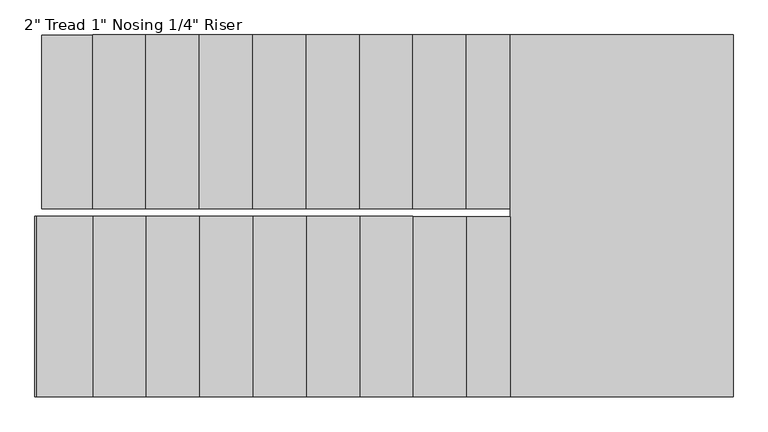
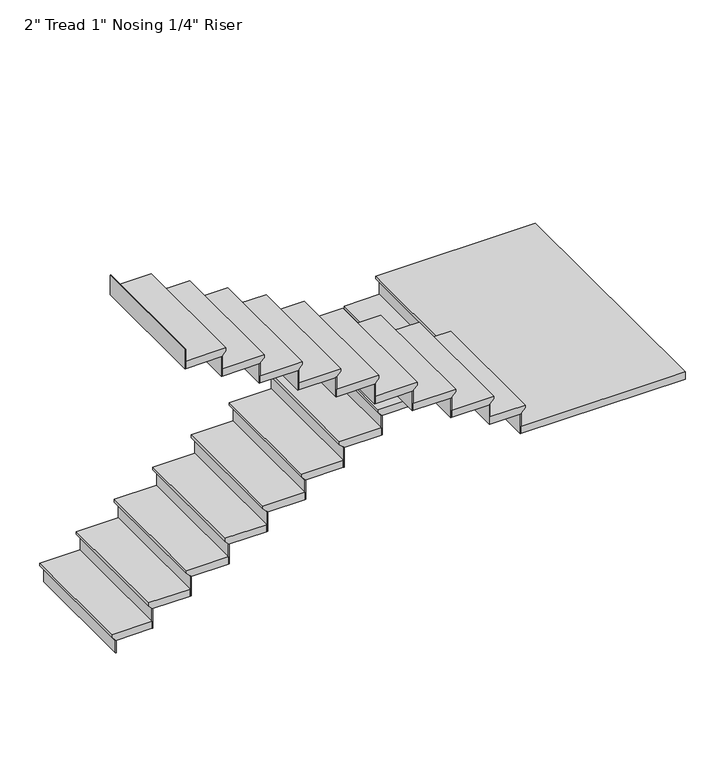
"""IFC4 building model written with IfcOpenShell, lengths in millimetres: stair flight geometry."""

from ifc_helpers import new_model, si_unit, origin, place, context, project, spatial, faceted_brep, source, transform, mapped, element, save


def stair_flight_b1286695(model_context):
    return source(origin(), model_context, "Body", "Brep", [
        faceted_brep([(1537.1941283, 180.9547293, 9262.11), (1537.1941283, 180.9547293, 9281.16), (1537.1941283, 1006.4547293, 9281.16), (1537.1941283, 1006.4547293, 9262.11), (1562.5941283, 180.9547293, 9236.71), (1562.5941283, 1006.4547293, 9236.71), (1804.8381368, 180.9547293, 9281.16), (1804.8381368, 1006.4547293, 9281.16), (1562.5941283, 1006.4547293, 9230.36), (1804.8381368, 1006.4547293, 9230.36), (1804.8381368, 180.9547293, 9230.36), (1562.5941283, 180.9547293, 9230.36)], [[[0, 1, 2, 3]], [[4, 0, 3, 5]], [[2, 1, 6, 7]], [[8, 9, 10, 11]], [[2, 7, 9, 8, 5, 3]], [[8, 11, 4, 5]], [[6, 1, 0, 4, 11, 10]], [[7, 6, 10, 9]]]),
        faceted_brep([(1562.5941283, 180.9547293, 9230.36), (1562.5941283, 180.9547293, 9144.0), (1568.9441283, 180.9547293, 9144.0), (1568.9441283, 180.9547293, 9230.36), (1562.5941283, 1006.4547293, 9230.36), (1568.9441283, 1006.4547293, 9230.36), (1568.9441283, 1006.4547293, 9144.0), (1562.5941283, 1006.4547293, 9144.0)], [[[0, 1, 2, 3]], [[4, 5, 6, 7]], [[1, 0, 4, 7]], [[2, 1, 7, 6]], [[3, 2, 6, 5]], [[0, 3, 5, 4]]]),
        faceted_brep([(1804.8381368, 180.9547293, 9367.52), (1804.8381368, 180.9547293, 9230.36), (1811.1881368, 180.9547293, 9230.36), (1811.1881368, 180.9547293, 9367.52), (1804.8381368, 1006.4547293, 9367.52), (1811.1881368, 1006.4547293, 9367.52), (1811.1881368, 1006.4547293, 9230.36), (1804.8381368, 1006.4547293, 9230.36)], [[[0, 1, 2, 3]], [[4, 5, 6, 7]], [[1, 0, 4, 7]], [[2, 1, 7, 6]], [[3, 2, 6, 5]], [[0, 3, 5, 4]]]),
        faceted_brep([(1779.4381368, 1006.4547293, 9418.32), (1779.4381368, 180.9547293, 9418.32), (2058.8381368, 180.9547293, 9418.32), (2058.8381368, 1006.4547293, 9418.32), (1804.8381368, 1006.4547293, 9367.52), (2058.8381368, 1006.4547293, 9367.52), (2058.8381368, 180.9547293, 9367.52), (1804.8381368, 180.9547293, 9367.52), (1804.8381368, 1006.4547293, 9373.87), (1779.4381368, 1006.4547293, 9399.27), (1804.8381368, 180.9547293, 9373.87), (1779.4381368, 180.9547293, 9399.27)], [[[0, 1, 2, 3]], [[4, 5, 6, 7]], [[0, 3, 5, 4, 8, 9]], [[4, 7, 10, 8]], [[2, 1, 11, 10, 7, 6]], [[3, 2, 6, 5]], [[11, 1, 0, 9]], [[10, 11, 9, 8]]]),
        faceted_brep([(2058.8381368, 180.9547293, 9504.68), (2058.8381368, 180.9547293, 9367.52), (2065.1881368, 180.9547293, 9367.52), (2065.1881368, 180.9547293, 9504.68), (2058.8381368, 1006.4547293, 9504.68), (2065.1881368, 1006.4547293, 9504.68), (2065.1881368, 1006.4547293, 9367.52), (2058.8381368, 1006.4547293, 9367.52)], [[[0, 1, 2, 3]], [[4, 5, 6, 7]], [[1, 0, 4, 7]], [[2, 1, 7, 6]], [[3, 2, 6, 5]], [[0, 3, 5, 4]]]),
        faceted_brep([(2033.4381368, 1006.4547293, 9555.48), (2033.4381368, 180.9547293, 9555.48), (2312.8381368, 180.9547293, 9555.48), (2312.8381368, 1006.4547293, 9555.48), (2058.8381368, 1006.4547293, 9504.68), (2312.8381368, 1006.4547293, 9504.68), (2312.8381368, 180.9547293, 9504.68), (2058.8381368, 180.9547293, 9504.68), (2058.8381368, 1006.4547293, 9511.03), (2033.4381368, 1006.4547293, 9536.43), (2058.8381368, 180.9547293, 9511.03), (2033.4381368, 180.9547293, 9536.43)], [[[0, 1, 2, 3]], [[4, 5, 6, 7]], [[0, 3, 5, 4, 8, 9]], [[4, 7, 10, 8]], [[2, 1, 11, 10, 7, 6]], [[3, 2, 6, 5]], [[11, 1, 0, 9]], [[10, 11, 9, 8]]]),
        faceted_brep([(2312.8381368, 180.9547293, 9641.84), (2312.8381368, 180.9547293, 9504.68), (2319.1881368, 180.9547293, 9504.68), (2319.1881368, 180.9547293, 9641.84), (2312.8381368, 1006.4547293, 9641.84), (2319.1881368, 1006.4547293, 9641.84), (2319.1881368, 1006.4547293, 9504.68), (2312.8381368, 1006.4547293, 9504.68)], [[[0, 1, 2, 3]], [[4, 5, 6, 7]], [[1, 0, 4, 7]], [[2, 1, 7, 6]], [[3, 2, 6, 5]], [[0, 3, 5, 4]]]),
        faceted_brep([(2287.4381368, 1006.4547293, 9692.64), (2287.4381368, 180.9547293, 9692.64), (2566.8381368, 180.9547293, 9692.64), (2566.8381368, 1006.4547293, 9692.64), (2312.8381368, 1006.4547293, 9641.84), (2566.8381368, 1006.4547293, 9641.84), (2566.8381368, 180.9547293, 9641.84), (2312.8381368, 180.9547293, 9641.84), (2312.8381368, 1006.4547293, 9648.19), (2287.4381368, 1006.4547293, 9673.59), (2312.8381368, 180.9547293, 9648.19), (2287.4381368, 180.9547293, 9673.59)], [[[0, 1, 2, 3]], [[4, 5, 6, 7]], [[0, 3, 5, 4, 8, 9]], [[4, 7, 10, 8]], [[2, 1, 11, 10, 7, 6]], [[3, 2, 6, 5]], [[11, 1, 0, 9]], [[10, 11, 9, 8]]]),
        faceted_brep([(2566.8381368, 180.9547293, 9779.0), (2566.8381368, 180.9547293, 9641.84), (2573.1881368, 180.9547293, 9641.84), (2573.1881368, 180.9547293, 9779.0), (2566.8381368, 1006.4547293, 9779.0), (2573.1881368, 1006.4547293, 9779.0), (2573.1881368, 1006.4547293, 9641.84), (2566.8381368, 1006.4547293, 9641.84)], [[[0, 1, 2, 3]], [[4, 5, 6, 7]], [[1, 0, 4, 7]], [[2, 1, 7, 6]], [[3, 2, 6, 5]], [[0, 3, 5, 4]]]),
        faceted_brep([(2541.4381368, 1006.4547293, 9829.8), (2541.4381368, 180.9547293, 9829.8), (2820.8381368, 180.9547293, 9829.8), (2820.8381368, 1006.4547293, 9829.8), (2566.8381368, 1006.4547293, 9779.0), (2820.8381368, 1006.4547293, 9779.0), (2820.8381368, 180.9547293, 9779.0), (2566.8381368, 180.9547293, 9779.0), (2566.8381368, 1006.4547293, 9785.35), (2541.4381368, 1006.4547293, 9810.75), (2566.8381368, 180.9547293, 9785.35), (2541.4381368, 180.9547293, 9810.75)], [[[0, 1, 2, 3]], [[4, 5, 6, 7]], [[0, 3, 5, 4, 8, 9]], [[4, 7, 10, 8]], [[2, 1, 11, 10, 7, 6]], [[3, 2, 6, 5]], [[11, 1, 0, 9]], [[10, 11, 9, 8]]]),
        faceted_brep([(2820.8381368, 180.9547293, 9916.16), (2820.8381368, 180.9547293, 9779.0), (2827.1881368, 180.9547293, 9779.0), (2827.1881368, 180.9547293, 9916.16), (2820.8381368, 1006.4547293, 9916.16), (2827.1881368, 1006.4547293, 9916.16), (2827.1881368, 1006.4547293, 9779.0), (2820.8381368, 1006.4547293, 9779.0)], [[[0, 1, 2, 3]], [[4, 5, 6, 7]], [[1, 0, 4, 7]], [[2, 1, 7, 6]], [[3, 2, 6, 5]], [[0, 3, 5, 4]]]),
        faceted_brep([(2795.4381368, 1006.4547293, 9966.96), (2795.4381368, 180.9547293, 9966.96), (3074.8381368, 180.9547293, 9966.96), (3074.8381368, 1006.4547293, 9966.96), (2820.8381368, 1006.4547293, 9916.16), (3074.8381368, 1006.4547293, 9916.16), (3074.8381368, 180.9547293, 9916.16), (2820.8381368, 180.9547293, 9916.16), (2820.8381368, 1006.4547293, 9922.51), (2795.4381368, 1006.4547293, 9947.91), (2820.8381368, 180.9547293, 9922.51), (2795.4381368, 180.9547293, 9947.91)], [[[0, 1, 2, 3]], [[4, 5, 6, 7]], [[0, 3, 5, 4, 8, 9]], [[4, 7, 10, 8]], [[2, 1, 11, 10, 7, 6]], [[3, 2, 6, 5]], [[11, 1, 0, 9]], [[10, 11, 9, 8]]]),
        faceted_brep([(3074.8381368, 180.9547293, 10053.32), (3074.8381368, 180.9547293, 9916.16), (3081.1881368, 180.9547293, 9916.16), (3081.1881368, 180.9547293, 10053.32), (3074.8381368, 1006.4547293, 10053.32), (3081.1881368, 1006.4547293, 10053.32), (3081.1881368, 1006.4547293, 9916.16), (3074.8381368, 1006.4547293, 9916.16)], [[[0, 1, 2, 3]], [[4, 5, 6, 7]], [[1, 0, 4, 7]], [[2, 1, 7, 6]], [[3, 2, 6, 5]], [[0, 3, 5, 4]]]),
        faceted_brep([(3049.4381368, 1006.4547293, 10104.12), (3049.4381368, 180.9547293, 10104.12), (3328.8381368, 180.9547293, 10104.12), (3328.8381368, 1006.4547293, 10104.12), (3074.8381368, 1006.4547293, 10053.32), (3328.8381368, 1006.4547293, 10053.32), (3328.8381368, 180.9547293, 10053.32), (3074.8381368, 180.9547293, 10053.32), (3074.8381368, 1006.4547293, 10059.67), (3049.4381368, 1006.4547293, 10085.07), (3074.8381368, 180.9547293, 10059.67), (3049.4381368, 180.9547293, 10085.07)], [[[0, 1, 2, 3]], [[4, 5, 6, 7]], [[0, 3, 5, 4, 8, 9]], [[4, 7, 10, 8]], [[2, 1, 11, 10, 7, 6]], [[3, 2, 6, 5]], [[11, 1, 0, 9]], [[10, 11, 9, 8]]]),
        faceted_brep([(3328.8381368, 180.9547293, 10190.48), (3328.8381368, 180.9547293, 10053.32), (3335.1881368, 180.9547293, 10053.32), (3335.1881368, 180.9547293, 10190.48), (3328.8381368, 1006.4547293, 10190.48), (3335.1881368, 1006.4547293, 10190.48), (3335.1881368, 1006.4547293, 10053.32), (3328.8381368, 1006.4547293, 10053.32)], [[[0, 1, 2, 3]], [[4, 5, 6, 7]], [[1, 0, 4, 7]], [[2, 1, 7, 6]], [[3, 2, 6, 5]], [[0, 3, 5, 4]]]),
        faceted_brep([(3303.4381368, 1006.4547293, 10241.28), (3303.4381368, 180.9547293, 10241.28), (3582.8381368, 180.9547293, 10241.28), (3582.8381368, 1006.4547293, 10241.28), (3328.8381368, 1006.4547293, 10190.48), (3582.8381368, 1006.4547293, 10190.48), (3582.8381368, 180.9547293, 10190.48), (3328.8381368, 180.9547293, 10190.48), (3328.8381368, 1006.4547293, 10196.83), (3303.4381368, 1006.4547293, 10222.23), (3328.8381368, 180.9547293, 10196.83), (3303.4381368, 180.9547293, 10222.23)], [[[0, 1, 2, 3]], [[4, 5, 6, 7]], [[0, 3, 5, 4, 8, 9]], [[4, 7, 10, 8]], [[2, 1, 11, 10, 7, 6]], [[3, 2, 6, 5]], [[11, 1, 0, 9]], [[10, 11, 9, 8]]]),
        faceted_brep([(3582.8381368, 180.9547293, 10327.64), (3582.8381368, 180.9547293, 10190.48), (3589.1881368, 180.9547293, 10190.48), (3589.1881368, 180.9547293, 10327.64), (3582.8381368, 1006.4547293, 10327.64), (3589.1881368, 1006.4547293, 10327.64), (3589.1881368, 1006.4547293, 10190.48), (3582.8381368, 1006.4547293, 10190.48)], [[[0, 1, 2, 3]], [[4, 5, 6, 7]], [[1, 0, 4, 7]], [[2, 1, 7, 6]], [[3, 2, 6, 5]], [[0, 3, 5, 4]]]),
        faceted_brep([(3557.4381368, 1006.4547293, 10378.44), (3557.4381368, 180.9547293, 10378.44), (3791.2648053, 180.9547293, 10378.44), (3791.2648053, 1006.4547293, 10378.44), (3582.8381368, 1006.4547293, 10327.64), (3791.2648053, 1006.4547293, 10327.64), (3791.2648053, 180.9547293, 10327.64), (3582.8381368, 180.9547293, 10327.64), (3582.8381368, 1006.4547293, 10333.99), (3557.4381368, 1006.4547293, 10359.39), (3582.8381368, 180.9547293, 10333.99), (3557.4381368, 180.9547293, 10359.39)], [[[0, 1, 2, 3]], [[4, 5, 6, 7]], [[0, 3, 5, 4, 8, 9]], [[4, 7, 10, 8]], [[2, 1, 11, 10, 7, 6]], [[3, 2, 6, 5]], [[11, 1, 0, 9]], [[10, 11, 9, 8]]]),
        faceted_brep([(3791.2648053, 180.9547293, 10464.8), (3791.2648053, 180.9547293, 10327.64), (3797.6148053, 180.9547293, 10327.64), (3797.6148053, 180.9547293, 10464.8), (3791.2648053, 1006.4547293, 10464.8), (3797.6148053, 1006.4547293, 10464.8), (3797.6148053, 1006.4547293, 10327.64), (3791.2648053, 1006.4547293, 10327.64)], [[[0, 1, 2, 3]], [[4, 5, 6, 7]], [[1, 0, 4, 7]], [[2, 1, 7, 6]], [[3, 2, 6, 5]], [[0, 3, 5, 4]]]),
        faceted_brep([(3740.4648053, -714.2964201, 10515.6), (4826.4941283, -714.2964201, 10515.6), (4826.4941283, 1006.4547293, 10515.6), (3765.8648053, 1006.4547293, 10515.6), (3765.8648053, 142.8547293, 10515.6), (3740.4648053, 142.8547293, 10515.6), (4826.4941283, -714.2964201, 10464.8), (3740.4648053, -714.2964201, 10464.8), (3740.4648053, 142.8547293, 10464.8), (3765.8648053, 142.8547293, 10464.8), (3765.8648053, 180.9547293, 10464.8), (3791.2648053, 180.9547293, 10464.8), (3791.2648053, 1006.4547293, 10464.8), (4826.4941283, 1006.4547293, 10464.8), (3791.2648053, 1006.4547293, 10471.15), (3765.8648053, 1006.4547293, 10496.55), (3791.2648053, 180.9547293, 10471.15), (3765.8648053, 180.9547293, 10496.55)], [[[0, 1, 2, 3, 4, 5]], [[6, 7, 8, 9, 10, 11, 12, 13]], [[1, 0, 7, 6]], [[2, 1, 6, 13]], [[3, 2, 13, 12, 14, 15]], [[12, 11, 16, 14]], [[11, 10, 17, 16]], [[4, 3, 15, 17, 10, 9]], [[5, 4, 9, 8]], [[0, 5, 8, 7]], [[15, 14, 16, 17]]]),
        faceted_brep([(3740.4648053, 142.8547293, 10601.96), (3740.4648053, 142.8547293, 10464.8), (3734.1148053, 142.8547293, 10464.8), (3734.1148053, 142.8547293, 10601.96), (3740.4648053, -714.2964201, 10601.96), (3734.1148053, -714.2964201, 10601.96), (3734.1148053, -714.2964201, 10464.8), (3740.4648053, -714.2964201, 10464.8)], [[[0, 1, 2, 3]], [[4, 5, 6, 7]], [[1, 0, 4, 7]], [[2, 1, 7, 6]], [[3, 2, 6, 5]], [[0, 3, 5, 4]]]),
        faceted_brep([(3765.8648053, -714.2964201, 10652.76), (3765.8648053, 142.8547293, 10652.76), (3532.0381368, 142.8547293, 10652.76), (3532.0381368, -714.2964201, 10652.76), (3740.4648053, -714.2964201, 10601.96), (3532.0381368, -714.2964201, 10601.96), (3532.0381368, 142.8547293, 10601.96), (3740.4648053, 142.8547293, 10601.96), (3740.4648053, -714.2964201, 10608.31), (3765.8648053, -714.2964201, 10633.71), (3740.4648053, 142.8547293, 10608.31), (3765.8648053, 142.8547293, 10633.71)], [[[0, 1, 2, 3]], [[4, 5, 6, 7]], [[0, 3, 5, 4, 8, 9]], [[4, 7, 10, 8]], [[2, 1, 11, 10, 7, 6]], [[3, 2, 6, 5]], [[11, 1, 0, 9]], [[10, 11, 9, 8]]]),
        faceted_brep([(3532.0381368, 142.8547293, 10739.12), (3532.0381368, 142.8547293, 10601.96), (3525.6881368, 142.8547293, 10601.96), (3525.6881368, 142.8547293, 10739.12), (3532.0381368, -714.2964201, 10739.12), (3525.6881368, -714.2964201, 10739.12), (3525.6881368, -714.2964201, 10601.96), (3532.0381368, -714.2964201, 10601.96)], [[[0, 1, 2, 3]], [[4, 5, 6, 7]], [[1, 0, 4, 7]], [[2, 1, 7, 6]], [[3, 2, 6, 5]], [[0, 3, 5, 4]]]),
        faceted_brep([(3557.4381368, -714.2964201, 10789.92), (3557.4381368, 142.8547293, 10789.92), (3278.0381368, 142.8547293, 10789.92), (3278.0381368, -714.2964201, 10789.92), (3532.0381368, -714.2964201, 10739.12), (3278.0381368, -714.2964201, 10739.12), (3278.0381368, 142.8547293, 10739.12), (3532.0381368, 142.8547293, 10739.12), (3532.0381368, -714.2964201, 10745.47), (3557.4381368, -714.2964201, 10770.87), (3532.0381368, 142.8547293, 10745.47), (3557.4381368, 142.8547293, 10770.87)], [[[0, 1, 2, 3]], [[4, 5, 6, 7]], [[0, 3, 5, 4, 8, 9]], [[4, 7, 10, 8]], [[2, 1, 11, 10, 7, 6]], [[3, 2, 6, 5]], [[11, 1, 0, 9]], [[10, 11, 9, 8]]]),
        faceted_brep([(3278.0381368, 142.8547293, 10876.28), (3278.0381368, 142.8547293, 10739.12), (3271.6881368, 142.8547293, 10739.12), (3271.6881368, 142.8547293, 10876.28), (3278.0381368, -714.2964201, 10876.28), (3271.6881368, -714.2964201, 10876.28), (3271.6881368, -714.2964201, 10739.12), (3278.0381368, -714.2964201, 10739.12)], [[[0, 1, 2, 3]], [[4, 5, 6, 7]], [[1, 0, 4, 7]], [[2, 1, 7, 6]], [[3, 2, 6, 5]], [[0, 3, 5, 4]]]),
        faceted_brep([(3303.4381368, -714.2964201, 10927.08), (3303.4381368, 142.8547293, 10927.08), (3024.0381368, 142.8547293, 10927.08), (3024.0381368, -714.2964201, 10927.08), (3278.0381368, -714.2964201, 10876.28), (3024.0381368, -714.2964201, 10876.28), (3024.0381368, 142.8547293, 10876.28), (3278.0381368, 142.8547293, 10876.28), (3278.0381368, -714.2964201, 10882.63), (3303.4381368, -714.2964201, 10908.03), (3278.0381368, 142.8547293, 10882.63), (3303.4381368, 142.8547293, 10908.03)], [[[0, 1, 2, 3]], [[4, 5, 6, 7]], [[0, 3, 5, 4, 8, 9]], [[4, 7, 10, 8]], [[2, 1, 11, 10, 7, 6]], [[3, 2, 6, 5]], [[11, 1, 0, 9]], [[10, 11, 9, 8]]]),
        faceted_brep([(3024.0381368, 142.8547293, 11013.44), (3024.0381368, 142.8547293, 10876.28), (3017.6881368, 142.8547293, 10876.28), (3017.6881368, 142.8547293, 11013.44), (3024.0381368, -714.2964201, 11013.44), (3017.6881368, -714.2964201, 11013.44), (3017.6881368, -714.2964201, 10876.28), (3024.0381368, -714.2964201, 10876.28)], [[[0, 1, 2, 3]], [[4, 5, 6, 7]], [[1, 0, 4, 7]], [[2, 1, 7, 6]], [[3, 2, 6, 5]], [[0, 3, 5, 4]]]),
        faceted_brep([(3049.4381368, -714.2964201, 11064.24), (3049.4381368, 142.8547293, 11064.24), (2770.0381368, 142.8547293, 11064.24), (2770.0381368, -714.2964201, 11064.24), (3024.0381368, -714.2964201, 11013.44), (2770.0381368, -714.2964201, 11013.44), (2770.0381368, 142.8547293, 11013.44), (3024.0381368, 142.8547293, 11013.44), (3024.0381368, -714.2964201, 11019.79), (3049.4381368, -714.2964201, 11045.19), (3024.0381368, 142.8547293, 11019.79), (3049.4381368, 142.8547293, 11045.19)], [[[0, 1, 2, 3]], [[4, 5, 6, 7]], [[0, 3, 5, 4, 8, 9]], [[4, 7, 10, 8]], [[2, 1, 11, 10, 7, 6]], [[3, 2, 6, 5]], [[11, 1, 0, 9]], [[10, 11, 9, 8]]]),
        faceted_brep([(2770.0381368, 142.8547293, 11150.6), (2770.0381368, 142.8547293, 11013.44), (2763.6881368, 142.8547293, 11013.44), (2763.6881368, 142.8547293, 11150.6), (2770.0381368, -714.2964201, 11150.6), (2763.6881368, -714.2964201, 11150.6), (2763.6881368, -714.2964201, 11013.44), (2770.0381368, -714.2964201, 11013.44)], [[[0, 1, 2, 3]], [[4, 5, 6, 7]], [[1, 0, 4, 7]], [[2, 1, 7, 6]], [[3, 2, 6, 5]], [[0, 3, 5, 4]]]),
        faceted_brep([(2795.4381368, -714.2964201, 11201.4), (2795.4381368, 142.8547293, 11201.4), (2516.0381368, 142.8547293, 11201.4), (2516.0381368, -714.2964201, 11201.4), (2770.0381368, -714.2964201, 11150.6), (2516.0381368, -714.2964201, 11150.6), (2516.0381368, 142.8547293, 11150.6), (2770.0381368, 142.8547293, 11150.6), (2770.0381368, -714.2964201, 11156.95), (2795.4381368, -714.2964201, 11182.35), (2770.0381368, 142.8547293, 11156.95), (2795.4381368, 142.8547293, 11182.35)], [[[0, 1, 2, 3]], [[4, 5, 6, 7]], [[0, 3, 5, 4, 8, 9]], [[4, 7, 10, 8]], [[2, 1, 11, 10, 7, 6]], [[3, 2, 6, 5]], [[11, 1, 0, 9]], [[10, 11, 9, 8]]]),
        faceted_brep([(2516.0381368, 142.8547293, 11287.76), (2516.0381368, 142.8547293, 11150.6), (2509.6881368, 142.8547293, 11150.6), (2509.6881368, 142.8547293, 11287.76), (2516.0381368, -714.2964201, 11287.76), (2509.6881368, -714.2964201, 11287.76), (2509.6881368, -714.2964201, 11150.6), (2516.0381368, -714.2964201, 11150.6)], [[[0, 1, 2, 3]], [[4, 5, 6, 7]], [[1, 0, 4, 7]], [[2, 1, 7, 6]], [[3, 2, 6, 5]], [[0, 3, 5, 4]]]),
        faceted_brep([(2541.4381368, -714.2964201, 11338.56), (2541.4381368, 142.8547293, 11338.56), (2262.0381368, 142.8547293, 11338.56), (2262.0381368, -714.2964201, 11338.56), (2516.0381368, -714.2964201, 11287.76), (2262.0381368, -714.2964201, 11287.76), (2262.0381368, 142.8547293, 11287.76), (2516.0381368, 142.8547293, 11287.76), (2516.0381368, -714.2964201, 11294.11), (2541.4381368, -714.2964201, 11319.51), (2516.0381368, 142.8547293, 11294.11), (2541.4381368, 142.8547293, 11319.51)], [[[0, 1, 2, 3]], [[4, 5, 6, 7]], [[0, 3, 5, 4, 8, 9]], [[4, 7, 10, 8]], [[2, 1, 11, 10, 7, 6]], [[3, 2, 6, 5]], [[11, 1, 0, 9]], [[10, 11, 9, 8]]]),
        faceted_brep([(2262.0381368, 142.8547293, 11424.92), (2262.0381368, 142.8547293, 11287.76), (2255.6881368, 142.8547293, 11287.76), (2255.6881368, 142.8547293, 11424.92), (2262.0381368, -714.2964201, 11424.92), (2255.6881368, -714.2964201, 11424.92), (2255.6881368, -714.2964201, 11287.76), (2262.0381368, -714.2964201, 11287.76)], [[[0, 1, 2, 3]], [[4, 5, 6, 7]], [[1, 0, 4, 7]], [[2, 1, 7, 6]], [[3, 2, 6, 5]], [[0, 3, 5, 4]]]),
        faceted_brep([(2287.4381368, -714.2964201, 11475.72), (2287.4381368, 142.8547293, 11475.72), (2008.0381368, 142.8547293, 11475.72), (2008.0381368, -714.2964201, 11475.72), (2262.0381368, -714.2964201, 11424.92), (2008.0381368, -714.2964201, 11424.92), (2008.0381368, 142.8547293, 11424.92), (2262.0381368, 142.8547293, 11424.92), (2262.0381368, -714.2964201, 11431.27), (2287.4381368, -714.2964201, 11456.67), (2262.0381368, 142.8547293, 11431.27), (2287.4381368, 142.8547293, 11456.67)], [[[0, 1, 2, 3]], [[4, 5, 6, 7]], [[0, 3, 5, 4, 8, 9]], [[4, 7, 10, 8]], [[2, 1, 11, 10, 7, 6]], [[3, 2, 6, 5]], [[11, 1, 0, 9]], [[10, 11, 9, 8]]]),
        faceted_brep([(2008.0381368, 142.8547293, 11562.08), (2008.0381368, 142.8547293, 11424.92), (2001.6881368, 142.8547293, 11424.92), (2001.6881368, 142.8547293, 11562.08), (2008.0381368, -714.2964201, 11562.08), (2001.6881368, -714.2964201, 11562.08), (2001.6881368, -714.2964201, 11424.92), (2008.0381368, -714.2964201, 11424.92)], [[[0, 1, 2, 3]], [[4, 5, 6, 7]], [[1, 0, 4, 7]], [[2, 1, 7, 6]], [[3, 2, 6, 5]], [[0, 3, 5, 4]]]),
        faceted_brep([(2033.4381368, -714.2964201, 11612.88), (2033.4381368, 142.8547293, 11612.88), (1754.0381368, 142.8547293, 11612.88), (1754.0381368, -714.2964201, 11612.88), (2008.0381368, -714.2964201, 11562.08), (1754.0381368, -714.2964201, 11562.08), (1754.0381368, 142.8547293, 11562.08), (2008.0381368, 142.8547293, 11562.08), (2008.0381368, -714.2964201, 11568.43), (2033.4381368, -714.2964201, 11593.83), (2008.0381368, 142.8547293, 11568.43), (2033.4381368, 142.8547293, 11593.83)], [[[0, 1, 2, 3]], [[4, 5, 6, 7]], [[0, 3, 5, 4, 8, 9]], [[4, 7, 10, 8]], [[2, 1, 11, 10, 7, 6]], [[3, 2, 6, 5]], [[11, 1, 0, 9]], [[10, 11, 9, 8]]]),
        faceted_brep([(1754.0381368, 142.8547293, 11699.24), (1754.0381368, 142.8547293, 11562.08), (1747.6881368, 142.8547293, 11562.08), (1747.6881368, 142.8547293, 11699.24), (1754.0381368, -714.2964201, 11699.24), (1747.6881368, -714.2964201, 11699.24), (1747.6881368, -714.2964201, 11562.08), (1754.0381368, -714.2964201, 11562.08)], [[[0, 1, 2, 3]], [[4, 5, 6, 7]], [[1, 0, 4, 7]], [[2, 1, 7, 6]], [[3, 2, 6, 5]], [[0, 3, 5, 4]]]),
        faceted_brep([(1511.7941283, 142.8547293, 11836.4), (1511.7941283, 142.8547293, 11699.24), (1505.4441283, 142.8547293, 11699.24), (1505.4441283, 142.8547293, 11836.4), (1511.7941283, -714.2964201, 11836.4), (1505.4441283, -714.2964201, 11836.4), (1505.4441283, -714.2964201, 11699.24), (1511.7941283, -714.2964201, 11699.24)], [[[0, 1, 2, 3]], [[4, 5, 6, 7]], [[1, 0, 4, 7]], [[2, 1, 7, 6]], [[3, 2, 6, 5]], [[0, 3, 5, 4]]]),
        faceted_brep([(1779.4381368, -714.2964201, 11750.04), (1779.4381368, 142.8547293, 11750.04), (1511.7941283, 142.8547293, 11750.04), (1511.7941283, -714.2964201, 11750.04), (1754.0381368, -714.2964201, 11699.24), (1511.7941283, -714.2964201, 11699.24), (1511.7941283, 142.8547293, 11699.24), (1754.0381368, 142.8547293, 11699.24), (1754.0381368, -714.2964201, 11705.59), (1779.4381368, -714.2964201, 11730.99), (1754.0381368, 142.8547293, 11705.59), (1779.4381368, 142.8547293, 11730.99)], [[[0, 1, 2, 3]], [[4, 5, 6, 7]], [[0, 3, 5, 4, 8, 9]], [[4, 7, 10, 8]], [[2, 1, 11, 10, 7, 6]], [[3, 2, 6, 5]], [[11, 1, 0, 9]], [[10, 11, 9, 8]]]),
    ])


if __name__ == "__main__":
    model = new_model("IFC4")
    model_context = context("Model", 3, world=origin())
    ifc_project = project(units=[si_unit("LENGTHUNIT", "METRE", prefix="MILLI")], contexts=[model_context])
    site = spatial("IfcSite", under=ifc_project)
    building = spatial("IfcBuilding", under=site)
    placement = place(None, origin())
    stair_flight_shape = stair_flight_b1286695(model_context)
    element("IfcStairFlight", 1, ObjectType="2\" Tread 1\" Nosing 1/4\" Riser", at=placement, inside=building, context=model_context, shape_type="MappedRepresentation", body=[
        mapped(stair_flight_shape, transform((0.0, 0.0, 0.0), x_axis=(1.0, 0.0, 0.0), y_axis=(0.0, 1.0, 0.0), z_axis=(0.0, 0.0, 1.0))),
    ])
    save(model, "model.ifc")
